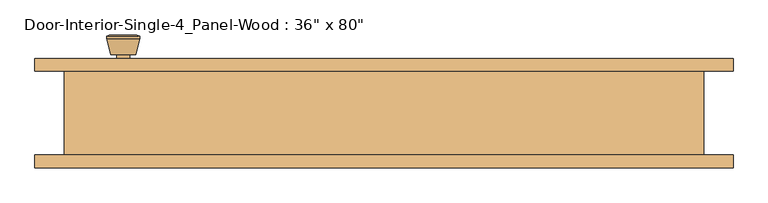
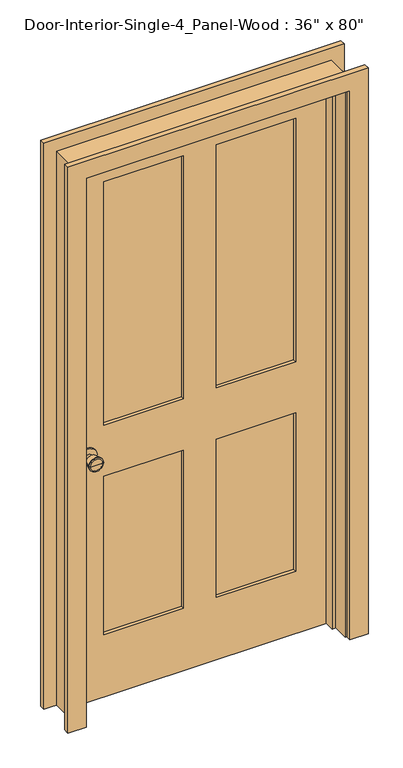
"""IFC4 building model written with IfcOpenShell, lengths in millimetres: door geometry."""

from ifc_helpers import new_model, si_unit, point, frame, frame_2d, origin, place, context, project, spatial, polyline, circle_curve, trimmed, segment, composite_curve, outline, extrude, faceted_brep, source, transform, mapped, element, save
from ifc_brep_helpers import plane_surface, cylinder_surface, revolved_surface, advanced_brep


def door_65ef8926(model_context):
    return source(origin(), model_context, "Body", "SolidModel", [
        advanced_brep(
        [(-393.7, 19.4, 914.4), (-383.7, 19.4, 914.4), (-403.7, 19.4, 914.4), (-373.2241324, -29.6, 914.4), (-393.7, -29.6, 914.4), (-414.1758676, -29.6, 914.4), (-368.7, -27.7721319, 914.4), (-418.7, -27.7721319, 914.4), (-368.7, -24.3084537, 914.4), (-418.7, -24.3084537, 914.4), (-375.063764, 0.4, 914.4), (-412.336236, 0.4, 914.4), (-383.7, 0.4, 914.4), (-403.7, 0.4, 914.4)],
        [
            (0, 1),
            (1, 2, circle_curve(frame((-393.7, 19.4, 914.4), z_axis=(0.0, 1.0, 0.0), x_axis=(-1.0, 0.0, 0.0)), 10.0)),
            (2, 0),
            (2, 1, circle_curve(frame((-393.7, 19.4, 914.4), z_axis=(0.0, 1.0, 0.0), x_axis=(-1.0, 0.0, 0.0)), 10.0)),
            (3, 4),
            (4, 5),
            (5, 3, circle_curve(frame((-393.7, -29.6, 914.4), z_axis=(0.0, -1.0, 0.0), x_axis=(-1.0, 0.0, 0.0)), 20.4758676)),
            (3, 5, circle_curve(frame((-393.7, -29.6, 914.4), z_axis=(0.0, -1.0, 0.0), x_axis=(-1.0, 0.0, 0.0)), 20.4758676)),
            (6, 3),
            (5, 7),
            (7, 6, circle_curve(frame((-393.7, -27.7721319, 914.4), z_axis=(0.0, -1.0, 0.0), x_axis=(-1.0, 0.0, 0.0)), 25.0)),
            (6, 7, circle_curve(frame((-393.7, -27.7721319, 914.4), z_axis=(0.0, -1.0, 0.0), x_axis=(-1.0, 0.0, 0.0)), 25.0)),
            (8, 6),
            (7, 9),
            (9, 8, circle_curve(frame((-393.7, -24.3084537, 914.4), z_axis=(0.0, -1.0, 0.0), x_axis=(-1.0, 0.0, 0.0)), 25.0)),
            (8, 9, circle_curve(frame((-393.7, -24.3084537, 914.4), z_axis=(0.0, -1.0, 0.0), x_axis=(-1.0, 0.0, 0.0)), 25.0)),
            (10, 8),
            (9, 11),
            (11, 10, circle_curve(frame((-393.7, 0.4, 914.4), z_axis=(0.0, -1.0, 0.0), x_axis=(-1.0, 0.0, 0.0)), 18.636236)),
            (10, 11, circle_curve(frame((-393.7, 0.4, 914.4), z_axis=(0.0, -1.0, 0.0), x_axis=(-1.0, 0.0, 0.0)), 18.636236)),
            (12, 10),
            (11, 13),
            (13, 12, circle_curve(frame((-393.7, 0.4, 914.4), z_axis=(0.0, -1.0, 0.0), x_axis=(-1.0, 0.0, 0.0)), 10.0)),
            (12, 13, circle_curve(frame((-393.7, 0.4, 914.4), z_axis=(0.0, -1.0, 0.0), x_axis=(-1.0, 0.0, 0.0)), 10.0)),
            (1, 12),
            (13, 2),
        ],
        [
            plane_surface(frame((-393.7, 19.4, 914.4), z_axis=(0.0, 1.0, 0.0), x_axis=(-1.0, 0.0, 0.0))),
            plane_surface(frame((-393.7, -29.6, 914.4), z_axis=(0.0, -1.0, 0.0), x_axis=(-1.0, 0.0, 0.0))),
            revolved_surface(polyline([(-414.1758676, -29.6, 914.4), (-418.7, -27.7721319, 914.4)]), (-393.7, 19.4, 914.4), (0.0, 1.0, 0.0)),
            cylinder_surface(frame((-393.7, 19.4, 914.4), z_axis=(0.0, 1.0, 0.0), x_axis=(-1.0, 0.0, 0.0)), 25.0),
            revolved_surface(polyline([(-418.7, -24.3084537, 914.4), (-412.336236, 0.4, 914.4)]), (-393.7, 19.4, 914.4), (0.0, 1.0, 0.0)),
            plane_surface(frame((-393.7, 0.4, 914.4), z_axis=(0.0, 1.0, 0.0), x_axis=(-1.0, 0.0, 0.0))),
            cylinder_surface(frame((-393.7, 19.4, 914.4), z_axis=(0.0, 1.0, 0.0), x_axis=(-1.0, 0.0, 0.0)), 10.0),
        ],
        [
            (0, [[1, 2, 3]]),
            (0, [[-3, 4, -1]]),
            (1, [[5, 6, 7]]),
            (1, [[-6, -5, 8]]),
            (2, [[9, -7, 10, 11]]),
            (2, [[-10, -8, -9, 12]]),
            (3, [[13, -11, 14, 15]]),
            (3, [[-14, -12, -13, 16]]),
            (4, [[17, -15, 18, 19]]),
            (4, [[-18, -16, -17, 20]]),
            (5, [[21, -19, 22, 23]]),
            (5, [[-22, -20, -21, 24]]),
            (6, [[25, -23, 26, -2]]),
            (6, [[-26, -24, -25, -4]]),
        ],
    ),
        extrude(outline(composite_curve([segment(trimmed(circle_curve(frame_2d((914.4, -393.7)), 30.0), [point((914.4, -423.7))], [point((914.4, -363.7))], False, "CARTESIAN"), True, "CONTINUOUS"), segment(trimmed(circle_curve(frame_2d((914.4, -393.7)), 30.0), [point((914.4, -363.7))], [point((914.4, -423.7))], False, "CARTESIAN"), True, "CONTINUOUS")], self_intersect=False)), frame((0.0, 19.4, 0.0), z_axis=(0.0, 1.0, 0.0), x_axis=(0.0, 0.0, 1.0)), (0.0, 0.0, 1.0), 6.0),
        advanced_brep(
        [(-393.7, 66.325, 914.4), (-403.7, 66.325, 914.4), (-383.7, 66.325, 914.4), (-373.2241324, 115.325, 914.4), (-414.1758676, 115.325, 914.4), (-393.7, 115.325, 914.4), (-368.7, 113.4971319, 914.4), (-418.7, 113.4971319, 914.4), (-368.7, 110.0334537, 914.4), (-418.7, 110.0334537, 914.4), (-375.063764, 85.325, 914.4), (-412.336236, 85.325, 914.4), (-383.7, 85.325, 914.4), (-403.7, 85.325, 914.4)],
        [
            (0, 1),
            (1, 2, circle_curve(frame((-393.7, 66.325, 914.4), z_axis=(0.0, -1.0, 0.0), x_axis=(-1.0, 0.0, 0.0)), 10.0)),
            (2, 0),
            (2, 1, circle_curve(frame((-393.7, 66.325, 914.4), z_axis=(0.0, -1.0, 0.0), x_axis=(-1.0, 0.0, 0.0)), 10.0)),
            (3, 4, circle_curve(frame((-393.7, 115.325, 914.4), z_axis=(0.0, 1.0, 0.0), x_axis=(-1.0, 0.0, 0.0)), 20.4758676)),
            (4, 5),
            (5, 3),
            (4, 3, circle_curve(frame((-393.7, 115.325, 914.4), z_axis=(0.0, 1.0, 0.0), x_axis=(-1.0, 0.0, 0.0)), 20.4758676)),
            (6, 7, circle_curve(frame((-393.7, 113.4971319, 914.4), z_axis=(0.0, 1.0, 0.0), x_axis=(-1.0, 0.0, 0.0)), 25.0)),
            (7, 4),
            (3, 6),
            (7, 6, circle_curve(frame((-393.7, 113.4971319, 914.4), z_axis=(0.0, 1.0, 0.0), x_axis=(-1.0, 0.0, 0.0)), 25.0)),
            (8, 9, circle_curve(frame((-393.7, 110.0334537, 914.4), z_axis=(0.0, 1.0, 0.0), x_axis=(-1.0, 0.0, 0.0)), 25.0)),
            (9, 7),
            (6, 8),
            (9, 8, circle_curve(frame((-393.7, 110.0334537, 914.4), z_axis=(0.0, 1.0, 0.0), x_axis=(-1.0, 0.0, 0.0)), 25.0)),
            (10, 11, circle_curve(frame((-393.7, 85.325, 914.4), z_axis=(0.0, 1.0, 0.0), x_axis=(-1.0, 0.0, 0.0)), 18.636236)),
            (11, 9),
            (8, 10),
            (11, 10, circle_curve(frame((-393.7, 85.325, 914.4), z_axis=(0.0, 1.0, 0.0), x_axis=(-1.0, 0.0, 0.0)), 18.636236)),
            (12, 13, circle_curve(frame((-393.7, 85.325, 914.4), z_axis=(0.0, 1.0, 0.0), x_axis=(-1.0, 0.0, 0.0)), 10.0)),
            (13, 11),
            (10, 12),
            (13, 12, circle_curve(frame((-393.7, 85.325, 914.4), z_axis=(0.0, 1.0, 0.0), x_axis=(-1.0, 0.0, 0.0)), 10.0)),
            (1, 13),
            (12, 2),
        ],
        [
            plane_surface(frame((-393.7, 66.325, 914.4), z_axis=(0.0, -1.0, 0.0), x_axis=(-1.0, 0.0, 0.0))),
            plane_surface(frame((-393.7, 115.325, 914.4), z_axis=(0.0, 1.0, 0.0), x_axis=(-1.0, 0.0, 0.0))),
            revolved_surface(polyline([(-414.1758676, 115.325, 914.4), (-418.7, 113.4971319, 914.4)]), (-393.7, 66.325, 914.4), (0.0, -1.0, 0.0)),
            cylinder_surface(frame((-393.7, 66.325, 914.4), z_axis=(0.0, -1.0, 0.0), x_axis=(-1.0, 0.0, 0.0)), 25.0),
            revolved_surface(polyline([(-418.7, 110.0334537, 914.4), (-412.336236, 85.325, 914.4)]), (-393.7, 66.325, 914.4), (0.0, -1.0, 0.0)),
            plane_surface(frame((-393.7, 85.325, 914.4), z_axis=(0.0, -1.0, 0.0), x_axis=(-1.0, 0.0, 0.0))),
            cylinder_surface(frame((-393.7, 66.325, 914.4), z_axis=(0.0, -1.0, 0.0), x_axis=(-1.0, 0.0, 0.0)), 10.0),
        ],
        [
            (0, [[1, 2, 3]]),
            (0, [[-3, 4, -1]]),
            (1, [[5, 6, 7]]),
            (1, [[8, -7, -6]]),
            (2, [[9, 10, -5, 11]]),
            (2, [[12, -11, -8, -10]]),
            (3, [[13, 14, -9, 15]]),
            (3, [[16, -15, -12, -14]]),
            (4, [[17, 18, -13, 19]]),
            (4, [[20, -19, -16, -18]]),
            (5, [[21, 22, -17, 23]]),
            (5, [[24, -23, -20, -22]]),
            (6, [[-2, 25, -21, 26]]),
            (6, [[-4, -26, -24, -25]]),
        ],
    ),
        extrude(outline(composite_curve([segment(trimmed(circle_curve(frame_2d((914.4, -393.7)), 30.0), [point((914.4, -423.7))], [point((914.4, -363.7))], False, "CARTESIAN"), True, "CONTINUOUS"), segment(trimmed(circle_curve(frame_2d((914.4, -393.7)), 30.0), [point((914.4, -363.7))], [point((914.4, -423.7))], False, "CARTESIAN"), True, "CONTINUOUS")], self_intersect=False)), frame((0.0, 60.325, 0.0), z_axis=(0.0, 1.0, 0.0), x_axis=(0.0, 0.0, 1.0)), (0.0, 0.0, 1.0), 6.0),
        faceted_brep([(482.6, 60.325, 0.0), (482.6, -66.675, 0.0), (457.2, -66.675, 0.0), (457.2, -9.525, 0.0), (444.5, -9.525, 0.0), (444.5, 25.4, 0.0), (457.2, 25.4, 0.0), (457.2, 60.325, 0.0), (482.6, 60.325, 2057.4), (482.6, -66.675, 2057.4), (-482.6, -66.675, 2057.4), (-482.6, -66.675, 0.0), (-457.2, -66.675, 0.0), (-457.2, -66.675, 2032.0), (457.2, -66.675, 2032.0), (457.2, -9.525, 2032.0), (-457.2, -9.525, 2032.0), (-457.2, -9.525, 0.0), (-444.5, -9.525, 0.0), (-444.5, -9.525, 2019.3), (444.5, -9.525, 2019.3), (444.5, 25.4, 2019.3), (-444.5, 25.4, 2019.3), (-444.5, 25.4, 0.0), (-457.2, 25.4, 0.0), (-457.2, 25.4, 2032.0), (457.2, 25.4, 2032.0), (457.2, 60.325, 2032.0), (-457.2, 60.325, 2032.0), (-457.2, 60.325, 0.0), (-482.6, 60.325, 0.0), (-482.6, 60.325, 2057.4)], [[[0, 1, 2, 3, 4, 5, 6, 7]], [[1, 0, 8, 9]], [[2, 1, 9, 10, 11, 12, 13, 14]], [[3, 2, 14, 15]], [[4, 3, 15, 16, 17, 18, 19, 20]], [[5, 4, 20, 21]], [[6, 5, 21, 22, 23, 24, 25, 26]], [[7, 6, 26, 27]], [[0, 7, 27, 28, 29, 30, 31, 8]], [[9, 8, 31, 10]], [[15, 14, 13, 16]], [[21, 20, 19, 22]], [[27, 26, 25, 28]], [[30, 29, 24, 23, 18, 17, 12, 11]], [[10, 31, 30, 11]], [[16, 13, 12, 17]], [[22, 19, 18, 23]], [[28, 25, 24, 29]]]),
        extrude(outline(polyline([(2032.0, -457.2), (0.0, -457.2), (0.0, 457.2), (2032.0, 457.2), (2032.0, -457.2)]), holes=[polyline([(1912.9375, 57.15), (1912.9375, 336.55), (1009.65, 336.55), (1009.65, 57.15), (1912.9375, 57.15)]), polyline([(1009.65, -57.15), (1009.65, -336.55), (1912.9375, -336.55), (1912.9375, -57.15), (1009.65, -57.15)]), polyline([(819.15, 57.15), (819.15, 336.55), (231.775, 336.55), (231.775, 57.15), (819.15, 57.15)]), polyline([(231.775, -57.15), (231.775, -336.55), (819.15, -336.55), (819.15, -57.15), (231.775, -57.15)])]), frame((0.0, 25.4, 0.0), z_axis=(0.0, 1.0, 0.0), x_axis=(0.0, 0.0, 1.0)), (0.0, 0.0, 1.0), 34.925),
        extrude(outline(polyline([(336.55, 37.0416667), (57.15, 37.0416667), (57.15, 48.6833333), (336.55, 48.6833333), (336.55, 37.0416667)])), frame((0.0, 0.0, 1009.65), z_axis=(0.0, 0.0, 1.0), x_axis=(1.0, 0.0, 0.0)), (0.0, 0.0, 1.0), 903.2875),
        extrude(outline(polyline([(-57.15, 37.0416667), (-336.55, 37.0416667), (-336.55, 48.6833333), (-57.15, 48.6833333), (-57.15, 37.0416667)])), frame((0.0, 0.0, 1009.65), z_axis=(0.0, 0.0, 1.0), x_axis=(1.0, 0.0, 0.0)), (0.0, 0.0, 1.0), 903.2875),
        extrude(outline(polyline([(336.55, 37.0416667), (57.15, 37.0416667), (57.15, 48.6833333), (336.55, 48.6833333), (336.55, 37.0416667)])), frame((0.0, 0.0, 231.775), z_axis=(0.0, 0.0, 1.0), x_axis=(1.0, 0.0, 0.0)), (0.0, 0.0, 1.0), 587.375),
        extrude(outline(polyline([(-57.15, 37.0416667), (-336.55, 37.0416667), (-336.55, 48.6833333), (-57.15, 48.6833333), (-57.15, 37.0416667)])), frame((0.0, 0.0, 231.775), z_axis=(0.0, 0.0, 1.0), x_axis=(1.0, 0.0, 0.0)), (0.0, 0.0, 1.0), 587.375),
        extrude(outline(polyline([(0.0, 463.55), (0.0, 527.05), (2101.85, 527.05), (2101.85, -527.05), (0.0, -527.05), (0.0, -463.55), (2038.35, -463.55), (2038.35, 463.55), (0.0, 463.55)])), frame((0.0, 60.325, 0.0), z_axis=(0.0, 1.0, 0.0), x_axis=(0.0, 0.0, 1.0)), (0.0, 0.0, 1.0), 19.05),
        extrude(outline(polyline([(0.0, 463.55), (0.0, 527.05), (2101.85, 527.05), (2101.85, -527.05), (0.0, -527.05), (0.0, -463.55), (2038.35, -463.55), (2038.35, 463.55), (0.0, 463.55)])), frame((0.0, -85.725, 0.0), z_axis=(0.0, 1.0, 0.0), x_axis=(0.0, 0.0, 1.0)), (0.0, 0.0, 1.0), 19.05),
    ])


if __name__ == "__main__":
    model = new_model("IFC4")
    model_context = context("Model", 3, world=origin())
    ifc_project = project(units=[si_unit("LENGTHUNIT", "METRE", prefix="MILLI")], contexts=[model_context])
    site = spatial("IfcSite", under=ifc_project)
    building = spatial("IfcBuilding", under=site)
    placement = place(None, origin())
    door_shape = door_65ef8926(model_context)
    element("IfcDoor", 1, ObjectType="Door-Interior-Single-4_Panel-Wood : 36\" x 80\"", at=placement, inside=building, context=model_context, shape_type="MappedRepresentation", body=[
        mapped(door_shape, transform((0.0, 0.0, 0.0), x_axis=(1.0, 0.0, 0.0), y_axis=(0.0, 1.0, 0.0), z_axis=(0.0, 0.0, 1.0))),
    ])
    save(model, "model.ifc")

# Revit data of these elements
# Type "Door-Interior-Single-4_Panel-Wood : 36\" x 80\""
#   Type Mark = "9"
#   Assembly Code = "C1020300"
#   Analytic Construction = "Wooden"
#   Top Rail = 0' - 4 11/16"
#   Thickness = 0' - 1 3/8"
#   Thermal Resistance (R) = 2.5876 (h·ft²·°F)/BTU
#   Swing Angle [instance default] = 90.00°
#   Stiles = 0' - 4 3/4"
#   Rough Width = 3' - 2"
#   Rough Height = 6' - 9"
#   Mullion = 0' - 4 1/2"
#   Lock Rail = 0' - 7 1/2"
#   Height = 6' - 8"
#   Width = 3' - 0"
#   Heat Transfer Coefficient (U) = 0.3865 BTU/(h·ft²·°F)
#   Bottom Rail = 0' - 9 1/8"
#   Trim Material = Cherry
#   Panel Material = Cherry
#   Frame Material = Cherry
#   Door Handle Material = Aluminum
#   Visual Light Transmittance = 0
#   Solar Heat Gain Coefficient = 0
#   Wall Closure = (empty or 0)
#   Function = (empty or 0)
# Element 1 (IfcDoor, "Door-Interior-Single-4_Panel-Wood : 36\" x 80\"")
#   Materials on its faces: "Cherry", "Aluminum"
# Materials
#   "Cherry": class "Wood", colour RGB 226 177 128, transparency 0, Description = "Prunus Serotina", Cost = 0
#   "Aluminum": class "Metal", colour RGB 247 247 247, transparency 0, Description = "Aluminum 6061", Cost = 0
